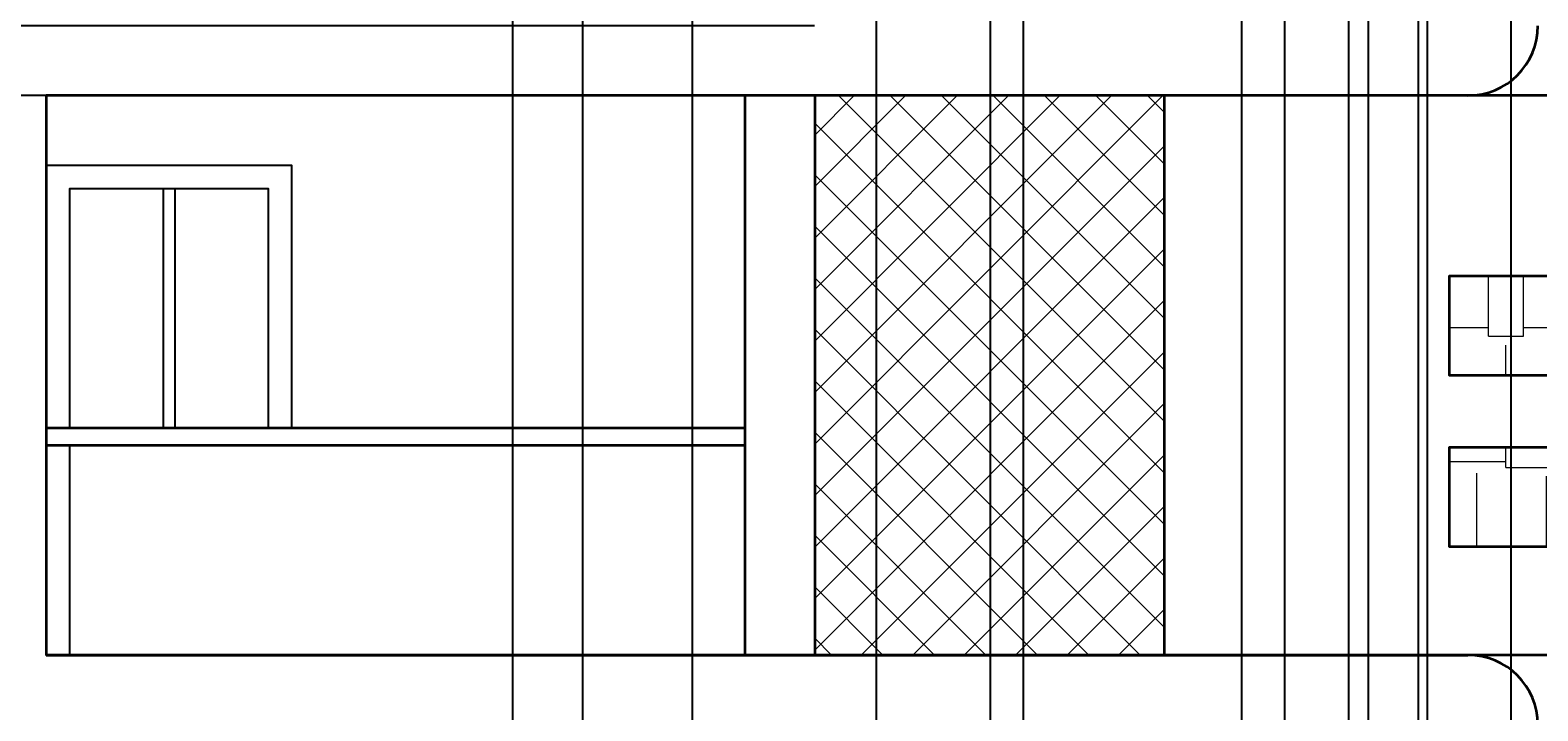
# Model space of a CAD drawing. Units: inches. Extents: x -15 to 605, y -220 to 570.
# Tile 8 of 10: x 138 to 397, y 222 to 339. Entities that reach past the tile are written whole.
import ezdxf

# ---------------------------------------------------------------- set-up
doc = ezdxf.new("R2010")
doc.units = ezdxf.units.IN
doc.header["$MEASUREMENT"] = 0
for name, color, linetype, lineweight in [('A-ANNO-DIMS', 2, 'Continuous', 18), ('A-DOOR', 4, 'Continuous', 25), ('A-ELEV', 7, 'Continuous', 35), ('A-ELEV-PATT', 8, 'Continuous', 13)]:
    doc.layers.add(name, color=color, linetype=linetype, lineweight=lineweight)
doc.styles.get("Standard").update_dxf_attribs({"font": 'arial.ttf'})
doc.dimstyles.get("Standard").update_dxf_attribs({"dimtxt": 0.18, "dimasz": 0.18, "dimexe": 0.18, "dimexo": 0.0625, "dimgap": 0.09, "dimtad": 0, "dimtih": 1, "dimtoh": 1, "dimdec": 4, "dimzin": 0, "dimdsep": 46, "dimtxsty": 'Standard', "dimcen": 0.09, "dimadec": 0, "dimazin": 0, "dimtfac": 1, "dimtdec": 4, "dimtofl": 0, "dimtmove": 0, "dimatfit": 3, "dimfxl": 1, "dimtolj": 1, "dimtzin": 0, "dimarcsym": 0})

# ---------------------------------------------------------------- blocks, each defined once
blk = doc.blocks.new('DOOR-ELEV')
for p, q in [((20.09, 80), (20.09, 39)), ((22.09, 80), (22.09, 39))]:
    blk.add_line(p, q)
for points in [[(42.18, 39), (42.18, 84), (0, 84), (0, 0), (42.18, 0)], [(38.18, 39), (38.18, 80), (4, 80), (4, 39)], [(4, 36), (4, 0)]]:
    blk.add_lwpolyline(points)
blk = doc.blocks.new('*D8')
at = {"layer": 'A-ANNO-DIMS', "color": 0, "lineweight": -2, "transparency": 16777216}
for p, q in [((23.99, 3.88), (23.99, 570.4)), ((24.17, 570.22), (263.7, 570.22)), ((503.81, 570.22), (264.28, 570.22)), ((503.99, 531.88), (503.99, 570.4))]:
    blk.add_line(p, q, dxfattribs=at)
at = {"layer": 'A-ANNO-DIMS', "color": 0, "transparency": 16777216}
for points in [[(24.17, 570.25), (24.17, 570.19), (23.99, 570.22)], [(503.81, 570.25), (503.81, 570.19), (503.99, 570.22)]]:
    blk.add_solid(points, dxfattribs=at)
at = {"layer": 'Defpoints', "color": 0, "transparency": 16777216}
for p in [(503.99, 570.22), (503.99, 531.82), (23.99, 3.82)]:
    blk.add_point(p, dxfattribs=at)
at = {"layer": 'A-ANNO-DIMS', "color": 0, "transparency": 16777216, "insert": (263.99, 570.22), "char_height": 0.18, "attachment_point": 5}
blk.add_mtext('\\A1;480', dxfattribs=at)
blk = doc.blocks.new('*D9')
at = {"layer": 'A-ANNO-DIMS', "color": 0, "lineweight": -2, "transparency": 16777216}
for p, q in [((503.92, 531.82), (-14.59, 531.82)), ((-14.41, 531.64), (-14.41, 208)), ((-14.41, -116), (-14.41, 207.64)), ((23.92, -116.18), (-14.59, -116.18))]:
    blk.add_line(p, q, dxfattribs=at)
at = {"layer": 'A-ANNO-DIMS', "color": 0, "transparency": 16777216}
for points in [[(-14.44, 531.64), (-14.38, 531.64), (-14.41, 531.82)], [(-14.44, -116), (-14.38, -116), (-14.41, -116.18)]]:
    blk.add_solid(points, dxfattribs=at)
at = {"layer": 'Defpoints', "color": 0, "transparency": 16777216}
for p in [(-14.41, 531.82), (503.99, 531.82), (23.99, -116.18)]:
    blk.add_point(p, dxfattribs=at)
at = {"layer": 'A-ANNO-DIMS', "color": 0, "transparency": 16777216, "insert": (-14.41, 207.82), "char_height": 0.18, "attachment_point": 5}
blk.add_mtext('\\A1;648', dxfattribs=at)
blk = doc.blocks.new('*D18')
at = {"layer": 'A-ANNO-DIMS', "color": 0, "lineweight": -2, "transparency": 16777216}
for p, q in [((23.99, 3.88), (23.99, 570.4)), ((24.17, 570.22), (143.44, 570.22)), ((263.64, 570.22), (144.37, 570.22)), ((263.82, 447.88), (263.82, 570.4))]:
    blk.add_line(p, q, dxfattribs=at)
at = {"layer": 'A-ANNO-DIMS', "color": 0, "transparency": 16777216}
for points in [[(24.17, 570.25), (24.17, 570.19), (23.99, 570.22)], [(263.64, 570.25), (263.64, 570.19), (263.82, 570.22)]]:
    blk.add_solid(points, dxfattribs=at)
at = {"layer": 'Defpoints', "color": 0, "transparency": 16777216}
for p in [(263.82, 570.22), (263.82, 447.82), (23.99, 3.82)]:
    blk.add_point(p, dxfattribs=at)
at = {"layer": 'A-ANNO-DIMS', "color": 0, "transparency": 16777216, "insert": (143.9, 570.22), "char_height": 0.18, "attachment_point": 5}
blk.add_mtext('\\A1;239.83', dxfattribs=at)
blk = doc.blocks.new('*D54')
at = {"layer": 'A-ANNO-DIMS', "color": 0, "lineweight": -2, "transparency": 16777216}
for p, q in [((63.91, -32.12), (63.91, 570.4)), ((64.09, 570.22), (142.07, 570.22)), ((220.96, 570.22), (142.98, 570.22)), ((221.14, -31.58), (221.14, 570.4))]:
    blk.add_line(p, q, dxfattribs=at)
at = {"layer": 'A-ANNO-DIMS', "color": 0, "transparency": 16777216}
for points in [[(64.09, 570.25), (64.09, 570.19), (63.91, 570.22)], [(220.96, 570.25), (220.96, 570.19), (221.14, 570.22)]]:
    blk.add_solid(points, dxfattribs=at)
at = {"layer": 'Defpoints', "color": 0, "transparency": 16777216}
for p in [(221.14, 570.22), (63.91, -32.18), (221.14, -31.64)]:
    blk.add_point(p, dxfattribs=at)
at = {"layer": 'A-ANNO-DIMS', "color": 0, "transparency": 16777216, "insert": (142.53, 570.22), "char_height": 0.18, "attachment_point": 5}
blk.add_mtext('\\A1;157.24', dxfattribs=at)
blk = doc.blocks.new('*D55')
at = {"layer": 'A-ANNO-DIMS', "color": 0, "lineweight": -2, "transparency": 16777216}
for p, q in [((221.14, -31.58), (221.14, 570.4)), ((221.32, 570.22), (226.93, 570.22)), ((232.96, 570.22), (227.35, 570.22)), ((233.14, -31.58), (233.14, 570.4))]:
    blk.add_line(p, q, dxfattribs=at)
at = {"layer": 'A-ANNO-DIMS', "color": 0, "transparency": 16777216}
for points in [[(221.32, 570.25), (221.32, 570.19), (221.14, 570.22)], [(232.96, 570.25), (232.96, 570.19), (233.14, 570.22)]]:
    blk.add_solid(points, dxfattribs=at)
at = {"layer": 'Defpoints', "color": 0, "transparency": 16777216}
for p in [(233.14, 570.22), (221.14, -31.64), (233.14, -31.64)]:
    blk.add_point(p, dxfattribs=at)
at = {"layer": 'A-ANNO-DIMS', "color": 0, "transparency": 16777216, "insert": (227.14, 570.22), "char_height": 0.18, "attachment_point": 5}
blk.add_mtext('\\A1;12', dxfattribs=at)
blk = doc.blocks.new('*D56')
at = {"layer": 'A-ANNO-DIMS', "color": 0, "lineweight": -2, "transparency": 16777216}
for p, q in [((233.14, -31.58), (233.14, 570.4)), ((233.32, 570.22), (298.47, 570.22)), ((364.53, 570.22), (299.38, 570.22)), ((364.71, -56.12), (364.71, 570.4))]:
    blk.add_line(p, q, dxfattribs=at)
at = {"layer": 'A-ANNO-DIMS', "color": 0, "transparency": 16777216}
for points in [[(233.32, 570.25), (233.32, 570.19), (233.14, 570.22)], [(364.53, 570.25), (364.53, 570.19), (364.71, 570.22)]]:
    blk.add_solid(points, dxfattribs=at)
at = {"layer": 'Defpoints', "color": 0, "transparency": 16777216}
for p in [(364.71, 570.22), (233.14, -31.64), (364.71, -56.18)]:
    blk.add_point(p, dxfattribs=at)
at = {"layer": 'A-ANNO-DIMS', "color": 0, "transparency": 16777216, "insert": (298.93, 570.22), "char_height": 0.18, "attachment_point": 5}
blk.add_mtext('\\A1;131.56', dxfattribs=at)
blk = doc.blocks.new('*D57')
at = {"layer": 'A-ANNO-DIMS', "color": 0, "lineweight": -2, "transparency": 16777216}
for p, q in [((364.71, -56.12), (364.71, 570.4)), ((364.89, 570.22), (370.5, 570.22)), ((376.53, 570.22), (370.92, 570.22)), ((376.71, -44.82), (376.71, 570.4))]:
    blk.add_line(p, q, dxfattribs=at)
at = {"layer": 'A-ANNO-DIMS', "color": 0, "transparency": 16777216}
for points in [[(364.89, 570.25), (364.89, 570.19), (364.71, 570.22)], [(376.53, 570.25), (376.53, 570.19), (376.71, 570.22)]]:
    blk.add_solid(points, dxfattribs=at)
at = {"layer": 'Defpoints', "color": 0, "transparency": 16777216}
for p in [(376.71, 570.22), (376.71, -44.88), (364.71, -56.18)]:
    blk.add_point(p, dxfattribs=at)
at = {"layer": 'A-ANNO-DIMS', "color": 0, "transparency": 16777216, "insert": (370.71, 570.22), "char_height": 0.18, "attachment_point": 5}
blk.add_mtext('\\A1;12', dxfattribs=at)
blk = doc.blocks.new('*D58')
at = {"layer": 'A-ANNO-DIMS', "color": 0, "lineweight": -2, "transparency": 16777216}
for p, q in [((376.71, -44.82), (376.71, 570.4)), ((376.89, 570.22), (419.58, 570.22)), ((462.92, 570.22), (420.23, 570.22)), ((463.1, -45.87), (463.1, 570.4))]:
    blk.add_line(p, q, dxfattribs=at)
at = {"layer": 'A-ANNO-DIMS', "color": 0, "transparency": 16777216}
for points in [[(376.89, 570.25), (376.89, 570.19), (376.71, 570.22)], [(462.92, 570.25), (462.92, 570.19), (463.1, 570.22)]]:
    blk.add_solid(points, dxfattribs=at)
at = {"layer": 'Defpoints', "color": 0, "transparency": 16777216}
for p in [(463.1, 570.22), (376.71, -44.88), (463.1, -45.94)]:
    blk.add_point(p, dxfattribs=at)
at = {"layer": 'A-ANNO-DIMS', "color": 0, "transparency": 16777216, "insert": (419.9, 570.22), "char_height": 0.18, "attachment_point": 5}
blk.add_mtext('\\A1;86.4', dxfattribs=at)
blk = doc.blocks.new('*D60')
at = {"layer": 'A-ANNO-DIMS', "color": 0, "lineweight": -2, "transparency": 16777216}
for p, q in [((346.37, -116.12), (346.37, 570.4)), ((346.55, 570.22), (349.67, 570.22)), ((353.57, 570.22), (350.45, 570.22)), ((353.75, -39.82), (353.75, 570.4))]:
    blk.add_line(p, q, dxfattribs=at)
at = {"layer": 'A-ANNO-DIMS', "color": 0, "transparency": 16777216}
for points in [[(346.55, 570.25), (346.55, 570.19), (346.37, 570.22)], [(353.57, 570.25), (353.57, 570.19), (353.75, 570.22)]]:
    blk.add_solid(points, dxfattribs=at)
at = {"layer": 'Defpoints', "color": 0, "transparency": 16777216}
for p in [(353.75, 570.22), (353.75, -39.88), (346.37, -116.18)]:
    blk.add_point(p, dxfattribs=at)
at = {"layer": 'A-ANNO-DIMS', "color": 0, "transparency": 16777216, "insert": (350.06, 570.22), "char_height": 0.18, "attachment_point": 5}
blk.add_mtext('\\A1;7.384', dxfattribs=at)
blk = doc.blocks.new('*D61')
at = {"layer": 'A-ANNO-DIMS', "color": 0, "lineweight": -2, "transparency": 16777216}
for p, q in [((353.75, -39.82), (353.75, 570.4)), ((353.93, 570.22), (360.55, 570.22)), ((367.95, 570.22), (361.33, 570.22)), ((368.13, -39.82), (368.13, 570.4))]:
    blk.add_line(p, q, dxfattribs=at)
at = {"layer": 'A-ANNO-DIMS', "color": 0, "transparency": 16777216}
for points in [[(353.93, 570.25), (353.93, 570.19), (353.75, 570.22)], [(367.95, 570.25), (367.95, 570.19), (368.13, 570.22)]]:
    blk.add_solid(points, dxfattribs=at)
at = {"layer": 'Defpoints', "color": 0, "transparency": 16777216}
for p in [(368.13, 570.22), (353.75, -39.88), (368.13, -39.88)]:
    blk.add_point(p, dxfattribs=at)
at = {"layer": 'A-ANNO-DIMS', "color": 0, "transparency": 16777216, "insert": (360.94, 570.22), "char_height": 0.18, "attachment_point": 5}
blk.add_mtext('\\A1;14.38', dxfattribs=at)
blk = doc.blocks.new('*D62')
at = {"layer": 'A-ANNO-DIMS', "color": 0, "lineweight": -2, "transparency": 16777216}
for p, q in [((378.23, -39.82), (378.23, 570.4)), ((378.41, 570.22), (385.04, 570.22)), ((392.43, 570.22), (385.81, 570.22)), ((392.61, -39.82), (392.61, 570.4))]:
    blk.add_line(p, q, dxfattribs=at)
at = {"layer": 'A-ANNO-DIMS', "color": 0, "transparency": 16777216}
for points in [[(378.41, 570.25), (378.41, 570.19), (378.23, 570.22)], [(392.43, 570.25), (392.43, 570.19), (392.61, 570.22)]]:
    blk.add_solid(points, dxfattribs=at)
at = {"layer": 'Defpoints', "color": 0, "transparency": 16777216}
for p in [(392.61, 570.22), (378.23, -39.88), (392.61, -39.88)]:
    blk.add_point(p, dxfattribs=at)
at = {"layer": 'A-ANNO-DIMS', "color": 0, "transparency": 16777216, "insert": (385.42, 570.22), "char_height": 0.18, "attachment_point": 5}
blk.add_mtext('\\A1;14.38', dxfattribs=at)
blk = doc.blocks.new('*D76')
at = {"layer": 'A-ANNO-DIMS', "color": 0, "lineweight": -2, "transparency": 16777216}
for p, q in [((272.92, 339.82), (-14.59, 339.82)), ((-14.41, 339.64), (-14.41, 334)), ((-14.41, 328), (-14.41, 333.64)), ((272.92, 327.82), (-14.59, 327.82))]:
    blk.add_line(p, q, dxfattribs=at)
at = {"layer": 'A-ANNO-DIMS', "color": 0, "transparency": 16777216}
for points in [[(-14.44, 339.64), (-14.38, 339.64), (-14.41, 339.82)], [(-14.44, 328), (-14.38, 328), (-14.41, 327.82)]]:
    blk.add_solid(points, dxfattribs=at)
at = {"layer": 'Defpoints', "color": 0, "transparency": 16777216}
for p in [(-14.41, 339.82), (272.99, 339.82), (272.99, 327.82)]:
    blk.add_point(p, dxfattribs=at)
at = {"layer": 'A-ANNO-DIMS', "color": 0, "transparency": 16777216, "insert": (-14.41, 333.82), "char_height": 0.18, "attachment_point": 5}
blk.add_mtext('\\A1;12', dxfattribs=at)
blk = doc.blocks.new('*D104')
at = {"layer": 'A-ANNO-DIMS', "color": 0, "lineweight": -2, "transparency": 16777216}
for p, q in [((251.99, -56.12), (251.99, 570.4)), ((252.17, 570.22), (267.39, 570.22)), ((283.41, 570.22), (268.18, 570.22)), ((283.59, -84.79), (283.59, 570.4))]:
    blk.add_line(p, q, dxfattribs=at)
at = {"layer": 'A-ANNO-DIMS', "color": 0, "transparency": 16777216}
for points in [[(252.17, 570.25), (252.17, 570.19), (251.99, 570.22)], [(283.41, 570.25), (283.41, 570.19), (283.59, 570.22)]]:
    blk.add_solid(points, dxfattribs=at)
at = {"layer": 'Defpoints', "color": 0, "transparency": 16777216}
for p in [(283.59, 570.22), (251.99, -56.18), (283.59, -84.86)]:
    blk.add_point(p, dxfattribs=at)
at = {"layer": 'A-ANNO-DIMS', "color": 0, "transparency": 16777216, "insert": (267.79, 570.22), "char_height": 0.18, "attachment_point": 5}
blk.add_mtext('\\A1;31.60', dxfattribs=at)
blk = doc.blocks.new('*D105')
at = {"layer": 'A-ANNO-DIMS', "color": 0, "lineweight": -2, "transparency": 16777216}
for p, q in [((283.59, -84.79), (283.59, 570.4)), ((283.77, 570.22), (292.92, 570.22)), ((302.99, 570.22), (293.84, 570.22)), ((303.17, -103.62), (303.17, 570.4))]:
    blk.add_line(p, q, dxfattribs=at)
at = {"layer": 'A-ANNO-DIMS', "color": 0, "transparency": 16777216}
for points in [[(283.77, 570.25), (283.77, 570.19), (283.59, 570.22)], [(302.99, 570.25), (302.99, 570.19), (303.17, 570.22)]]:
    blk.add_solid(points, dxfattribs=at)
at = {"layer": 'Defpoints', "color": 0, "transparency": 16777216}
for p in [(303.17, 570.22), (283.59, -84.86), (303.17, -103.68)]:
    blk.add_point(p, dxfattribs=at)
at = {"layer": 'A-ANNO-DIMS', "color": 0, "transparency": 16777216, "insert": (293.38, 570.22), "char_height": 0.18, "attachment_point": 5}
blk.add_mtext('\\A1;19.585', dxfattribs=at)
blk = doc.blocks.new('*D106')
at = {"layer": 'A-ANNO-DIMS', "color": 0, "lineweight": -2, "transparency": 16777216}
for p, q in [((303.17, -103.62), (303.17, 570.4)), ((303.35, 570.22), (305.62, 570.22)), ((308.68, 570.22), (306.41, 570.22)), ((308.86, -79.16), (308.86, 570.4))]:
    blk.add_line(p, q, dxfattribs=at)
at = {"layer": 'A-ANNO-DIMS', "color": 0, "transparency": 16777216}
for points in [[(303.35, 570.25), (303.35, 570.19), (303.17, 570.22)], [(308.68, 570.25), (308.68, 570.19), (308.86, 570.22)]]:
    blk.add_solid(points, dxfattribs=at)
at = {"layer": 'Defpoints', "color": 0, "transparency": 16777216}
for p in [(308.86, 570.22), (308.86, -79.22), (303.17, -103.68)]:
    blk.add_point(p, dxfattribs=at)
at = {"layer": 'A-ANNO-DIMS', "color": 0, "transparency": 16777216, "insert": (306.02, 570.22), "char_height": 0.18, "attachment_point": 5}
blk.add_mtext('\\A1;5.689', dxfattribs=at)

msp = doc.modelspace()

# ---------------------------------------------------------------- hatches: boundary and pattern name
at = {"layer": 'A-ELEV-PATT'}
h = msp.add_hatch(dxfattribs=at)
h.set_pattern_fill('AR-RSHKE', color=256, scale=2)
h.set_pattern_definition([(0, (-191.319, 0), (51, 24), [12, -10, 14, -6, 18, -8]), (0, (-179.319, 1), (51, 24), [10, -38, 8, -12]), (0, (-155.319, -1.5), (51, 24), [6, -62]), (90, (-191.319, 0), (-17, 24), [23, -73]), (90, (-179.319, 0), (-17, 24), [22.5, -73.5]), (90, (-169.319, 0), (-17, 24), [21, -75]), (90, (-155.319, -1.5), (-17, 24), [23, -73]), (90, (-149.319, -1.5), (-17, 24), [23, -73]), (90, (-131.319, 0), (-17, 24), [22, -74])])
h.paths.add_polyline_path([(491.9872, 80.9192), (382.0304, 80.9192), (382.0304, 63.8187), (491.9872, 63.8187)])
h.paths.add_polyline_path([(491.9872, 51.4763), (382.0304, 51.4763), (382.0304, 34.3758), (491.9872, 34.3758)])
h.paths.add_polyline_path([(433.9097, 207.1093), (417.1672, 207.1093), (417.1672, 136.5115), (433.9097, 136.5115)])
h.paths.add_polyline_path([(466.4098, 207.1093), (451.1446, 207.1093), (451.1446, 136.5115), (466.4098, 136.5115)])
h.paths.add_polyline_path([(491.9872, 296.9192), (382.0304, 296.9192), (382.0304, 279.8187), (491.9872, 279.8187)])
h.paths.add_polyline_path([(491.9872, 267.4763), (382.0304, 267.4763), (382.0304, 250.3758), (491.9872, 250.3758)])
h.paths.add_polyline_path([(433.9097, 423.1093), (417.1672, 423.1093), (417.1672, 352.5115), (433.9097, 352.5115)])
h.paths.add_polyline_path([(466.4098, 423.1093), (451.1446, 423.1093), (451.1446, 352.5115), (466.4098, 352.5115)])
h = msp.add_hatch(dxfattribs=at)
h.set_pattern_fill('ANSI37', color=256, scale=50)
h.set_pattern_definition([(45, (0, 216), (-4.41942, 4.41942), []), (135, (0, 216), (-4.41942, -4.41942), [])])
h.paths.add_polyline_path([(332.9872, 327.8187), (272.9872, 327.8187), (272.9872, 231.8187), (332.9872, 231.8187)])

# ---------------------------------------------------------------- linework, layer by layer
at = {"layer": 'A-ELEV'}
for p, q in [((491.9872, 327.8187), (140.9872, 327.8187)), ((140.9872, 327.8187), (140.9872, 231.8187)), ((260.9872, 327.8187), (260.9872, 231.8187)), ((272.9872, 327.8187), (272.9872, 231.8187)), ((332.9872, 327.8187), (332.9872, 231.8187)), ((491.9872, 231.8187), (140.9872, 231.8187)), ((140.9872, 231.8187), (212.3003, 231.8187)), ((212.3003, 231.8187), (260.9872, 231.8187)), ((260.9872, 231.8187), (385.1921, 231.8187))]:
    msp.add_line(p, q, dxfattribs=at)
for points in [[(491.9872, 279.8187), (382.0304, 279.8187), (382.0304, 296.9192), (491.9872, 296.9192)], [(491.9872, 250.3758), (382.0304, 250.3758), (382.0304, 267.4763), (491.9872, 267.4763)]]:
    msp.add_lwpolyline(points, close=True, dxfattribs=at)
for points in [[(140.9872, 270.8187), (212.3003, 270.8187), (260.9872, 270.8187)], [(140.9872, 267.8187), (212.3003, 267.8187), (260.9872, 267.8187)]]:
    msp.add_lwpolyline(points, dxfattribs=at)
for centre, start, end in [((385.1921, 339.8187), 270, 0), ((385.1921, 219.8187), 0, 90)]:
    msp.add_arc(centre, 12, start, end, dxfattribs=at)

# ---------------------------------------------------------------- block references
at = {"layer": 'A-DOOR'}
msp.add_blockref('DOOR-ELEV', (140.987, 231.819), dxfattribs=at)

# ---------------------------------------------------------------- dimensions: what is measured, and where the dimension line sits
at = {"layer": 'A-ANNO-DIMS'}
for base, p1, p2, override, picture, middle in [((503.9872, 570.2187), (23.9872, 3.8187), (503.9872, 531.8187), {"dimdec": 0, "dimlfac": 1, "dimrnd": 0, "dimzin": 0, "dimdsep": 46, "dimlunit": 2}, '*D8', (263.9872, 570.2187)), ((263.8163, 570.2187), (23.9872, 3.8187), (263.8163, 447.8187), {"dimdec": 2, "dimlfac": 1, "dimrnd": 0, "dimzin": 0, "dimdsep": 46, "dimlunit": 2}, '*D18', (143.9018, 570.2187)), ((221.1439, 570.2187), (63.9067, -32.1813), (221.1439, -31.6396), {"dimdec": 2, "dimlfac": 1, "dimrnd": 0, "dimzin": 0, "dimdsep": 46, "dimlunit": 2}, '*D54', (142.5253, 570.2187)), ((233.1439, 570.2187), (221.1439, -31.6396), (233.1439, -31.6396), {"dimdec": 0, "dimlfac": 1, "dimrnd": 0, "dimzin": 0, "dimdsep": 46, "dimlunit": 2}, '*D55', (227.1439, 570.2187)), ((364.7066, 570.2187), (233.1439, -31.6396), (364.7066, -56.1813), {"dimdec": 2, "dimlfac": 1, "dimrnd": 0, "dimzin": 0, "dimdsep": 46, "dimlunit": 2}, '*D56', (298.9252, 570.2187)), ((283.5871, 570.2187), (251.9872, -56.1813), (283.5871, -84.8572), {"dimdec": 2, "dimlfac": 1, "dimrnd": 0, "dimzin": 0, "dimdsep": 46, "dimlunit": 2}, '*D104', (267.7872, 570.2187)), ((303.1719, 570.2187), (283.5871, -84.8572), (303.1719, -103.6786), {"dimdec": 3, "dimlfac": 1, "dimrnd": 0, "dimzin": 0, "dimdsep": 46, "dimlunit": 2}, '*D105', (293.3795, 570.2187)), ((308.8611, 570.2187), (303.1719, -103.6786), (308.8611, -79.2202), {"dimdec": 3, "dimlfac": 1, "dimrnd": 0, "dimzin": 0, "dimdsep": 46, "dimlunit": 2}, '*D106', (306.0165, 570.2187)), ((353.7501, 570.2187), (346.3663, -116.1813), (353.7501, -39.8843), {"dimdec": 3, "dimlfac": 1, "dimrnd": 0, "dimzin": 0, "dimdsep": 46, "dimlunit": 2}, '*D60', (350.0582, 570.2187)), ((368.1292, 570.2187), (353.7501, -39.8843), (368.1292, -39.8843), {"dimdec": 2, "dimlfac": 1, "dimrnd": 0, "dimzin": 0, "dimdsep": 46, "dimlunit": 2}, '*D61', (360.9397, 570.2187)), ((376.7066, 570.2187), (364.7066, -56.1813), (376.7066, -44.8803), {"dimdec": 0, "dimlfac": 1, "dimrnd": 0, "dimzin": 0, "dimdsep": 46, "dimlunit": 2}, '*D57', (370.7066, 570.2187)), ((463.1032, 570.2187), (376.7066, -44.8803), (463.1032, -45.9373), {"dimdec": 1, "dimlfac": 1, "dimrnd": 0, "dimzin": 0, "dimdsep": 46, "dimlunit": 2}, '*D58', (419.9049, 570.2187)), ((392.6125, 570.2187), (378.2334, -39.8843), (392.6125, -39.8843), {"dimdec": 2, "dimlfac": 1, "dimrnd": 0, "dimzin": 0, "dimdsep": 46, "dimlunit": 2}, '*D62', (385.423, 570.2187))]:
    dim = msp.add_linear_dim(base=base, p1=p1, p2=p2, dimstyle='Standard', override=override, dxfattribs=at)
    dim.commit()
    dim.dimension.update_dxf_attribs({"geometry": picture, "text_midpoint": middle})
for base, p1, p2, picture, middle in [((-14.4128, 531.8187), (23.9872, -116.1813), (503.9872, 531.8187), '*D9', (-14.4128, 207.8187)), ((-14.4128, 339.8187), (272.9872, 327.8187), (272.9872, 339.8187), '*D76', (-14.4128, 333.8187))]:
    dim = msp.add_linear_dim(base=base, p1=p1, p2=p2, angle=90, dimstyle='Standard', override={"dimdec": 0, "dimlfac": 1, "dimrnd": 0, "dimzin": 0, "dimdsep": 46, "dimlunit": 2}, dxfattribs=at)
    dim.commit()
    dim.dimension.update_dxf_attribs({"geometry": picture, "text_midpoint": middle})

doc.saveas('drawing.dxf')
